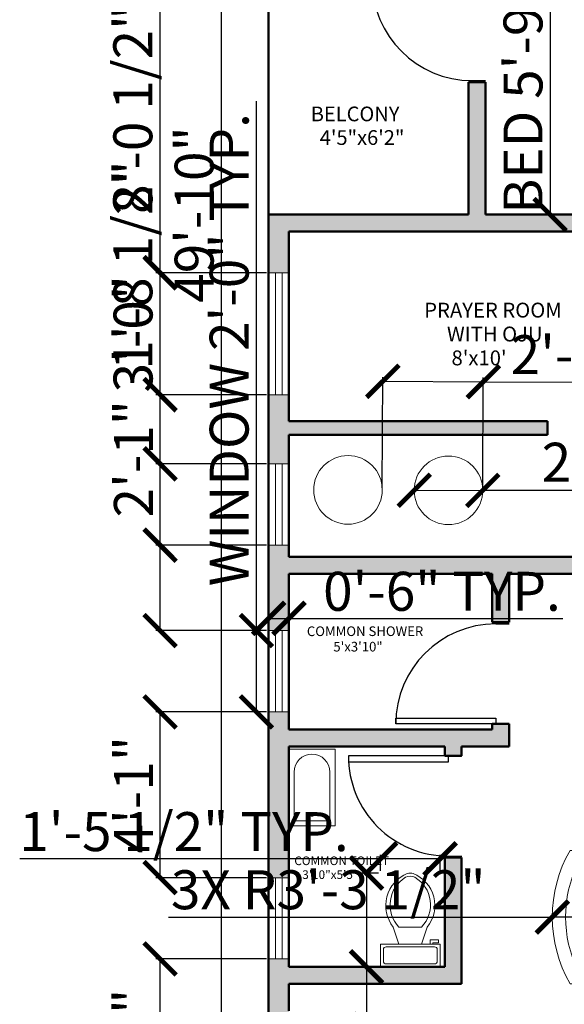
# Model space of a CAD drawing. Units: inches. Extents: x 3147 to 3847, y 1414 to 2207.
# Tile 2 of 7: x 3276 to 3437, y 1561 to 1852. Entities that reach past the tile are written whole.
import ezdxf

# ---------------------------------------------------------------- set-up
doc = ezdxf.new("R2010")
doc.units = ezdxf.units.IN
for name, color, linetype, lineweight in [('A-ANNO-DIMS', 2, 'Continuous', 18), ('A-AREA-IDEN', 7, 'Continuous', 18), ('A-DOOR', 3, 'Continuous', 25), ('A-FLOR-FIXT', 9, 'Continuous', 18), ('A-FURN', 8, 'Continuous', 18), ('A-GLAZ', 4, 'Continuous', 18), ('A-WALL', 7, 'Continuous', 50)]:
    doc.layers.add(name, color=color, linetype=linetype, lineweight=lineweight)
doc.layers.add('A-WALL-PATT', color=18, linetype='Continuous', lineweight=13, true_color=0x000000)
doc.styles.get("Standard").update_dxf_attribs({"font": 'arial.ttf'})
doc.dimstyles.new('ISO-25', dxfattribs={"dimtxt": 11.5, "dimasz": 9.5, "dimexe": 1.25, "dimexo": 0.625, "dimtad": 1, "dimdec": 0, "dimlunit": 3, "dimtxsty": 'Standard', "dimblk": 'ARCHTICK', "dimcen": 2.5, "dimadec": 0, "dimazin": 0, "dimtfac": 1, "dimtdec": 0, "dimtmove": 0, "dimatfit": 3, "dimfxl": 1, "dimarcsym": 0})

# ---------------------------------------------------------------- blocks, each defined once
blk = doc.blocks.new('*U3')
for p, q in [((0, 0), (0, -100)), ((750, 0), (750, -100))]:
    blk.add_line(p, q)
blk.add_lwpolyline([(0, 0), (0, 750), (43.75, 750), (43.75, 0)], close=True)
blk.add_arc((0, 0), 750, 0, 90)
blk = doc.blocks.new('*U4')
for p, q in [((-750, 0), (-750, -100)), ((0, 0), (0, -100))]:
    blk.add_line(p, q)
blk.add_lwpolyline([(0, 0), (0, 750), (-43.75, 750), (-43.75, 0)], close=True)
blk.add_arc((0, 0), 750, 90, 180)
blk = doc.blocks.new('Bath Tub - 26 x 60 in.')
for p, q in [((8, -18), (10, -18)), ((9, -17), (9, -19))]:
    blk.add_line(p, q)
blk.add_lwpolyline([(0, -36), (0, 0), (60, 0), (60, -36)], close=True)
for points in [[(4, -30), (4, -6)], [(6, -4), (42, -4)], [(42, -32), (6, -32)]]:
    blk.add_lwpolyline(points)
for radius in [1.5, 1]:
    blk.add_circle((9, -18), radius)
for centre, radius, start, end in [((5.75, -5.75), 1.77, 81.8699, 188.1301), ((42, -18), 14, 270, 90), ((5.75, -30.25), 1.77, 171.8699, 278.1301)]:
    blk.add_arc(centre, radius, start, end)
blk = doc.blocks.new('Toilet - top')
for p, q in [((9.5, -6), (9.5, -2)), ((-10, -8.5), (-8, -8.5)), ((-10, -9.5), (-10, -8.5)), ((-7, -9.5), (-10, -9.5)), ((-8, -8.5), (-8, -8)), ((-7, -8), (-7, -9.5)), ((-4, -8), (-6, -14)), ((4, -8), (6, -14)), ((4, -14), (-4, -14))]:
    blk.add_line(p, q)
blk.add_lwpolyline([(10.5, -8), (10.5, 0), (-10.5, 0), (-10.5, -8)], close=True)
for points in [[(-9.5, -2), (-9.5, -6)], [(8.5, -1), (-8.5, -1)], [(-8.5, -7), (8.5, -7)]]:
    blk.add_lwpolyline(points)
for centre, radius, start, end in [((-8.62, -1.88), 0.884, 81.8699, 188.1301), ((8.62, -1.88), 0.884, 351.8699, 98.1301), ((-8.62, -6.12), 0.884, 171.8699, 278.1301), ((8.62, -6.12), 0.884, 261.8699, 8.1301), ((3.52, -21.58), 12.17, 141.4691, 247.9714), ((4.2, -21.82), 11.33, 136.3677, 238.9468), ((-3.52, -21.58), 12.17, 292.0284, 38.5307), ((-4.2, -21.82), 11.33, 301.053, 43.6321), ((0, -27.88), 4, 245.7318, 294.2682), ((0, -29), 4, 254.8605, 285.1395)]:
    blk.add_arc(centre, radius, start, end)
blk = doc.blocks.new('Sofa - Roundback Loveseat 5 ft.')
for p, q in [((0, -32.44198), (0, -5.99998)), ((-24, -33.99998), (-24, -11.46958)), ((24.00004, -33.99998), (24.00004, -11.46958)), ((-23.9998, -13.38178), (23.99986, -13.38178)), ((-24, -32.44198), (24.00004, -32.44198))]:
    blk.add_line(p, q)
for points in [[(-24, -33.99998), (-30, -33.99998), (-30, -7.99998)], [(30.00004, -7.99998), (30.00004, -33.99998), (24.00004, -33.99998)]]:
    blk.add_lwpolyline(points)
for centre, radius, start, end in [((0, -60.24998), 60.24998, 60.13715, 119.8628), ((0, -61.38438), 55.38444, 64.32083, 115.6792)]:
    blk.add_arc(centre, radius, start, end)
blk = doc.blocks.new('_ArchTick')
at = {"color": 0, "linetype": 'ByBlock', "const_width": 0.15}
blk.add_lwpolyline([(-0.5, -0.5), (0.5, 0.5)], dxfattribs=at)
blk = doc.blocks.new('*D22')
at = {"layer": 'A-ANNO-DIMS', "color": 0, "lineweight": -2, "transparency": 16777216}
for p, q in [((3349.14, 2093.05), (3334.5, 2093.05)), ((3335.75, 2093.05), (3335.75, 1495.05)), ((3349.14, 1495.05), (3334.5, 1495.05))]:
    blk.add_line(p, q, dxfattribs=at)
at = {"layer": 'Defpoints', "color": 0, "transparency": 16777216}
for p in [(3349.76, 2093.05), (3335.75, 1495.05), (3349.76, 1495.05)]:
    blk.add_point(p, dxfattribs=at)
at = {"layer": 'A-ANNO-DIMS', "color": 0, "lineweight": -2, "transparency": 16777216, "xscale": 9.5, "yscale": 9.5, "zscale": 9.5}
for p, rotation in [((3335.75, 2093.05), 90), ((3335.75, 1495.05), 270)]:
    blk.add_blockref('_ArchTick', p, dxfattribs=dict(at, rotation=rotation))
at = {"layer": 'A-ANNO-DIMS', "color": 0, "transparency": 16777216, "insert": (3329.25, 1794.05), "char_height": 11.5, "attachment_point": 5, "rotation": 90}
blk.add_mtext('49\'-10"', dxfattribs=at)
blk = doc.blocks.new('WIN-24IN')
for p, q in [((6, 24), (0, 24)), ((2, 0), (2, 24)), ((4, 0), (4, 24)), ((6, 0), (0, 0))]:
    blk.add_line(p, q)
blk = doc.blocks.new('OJU-ROUND-FIXTURE')
blk.add_circle((10.13, 10.13), 10.13)
blk = doc.blocks.new('*D27')
at = {"layer": 'A-ANNO-DIMS', "color": 0, "lineweight": -2, "transparency": 16777216}
for p, q in [((3346.16, 1671.27), (3346.16, 1827.54)), ((3349.14, 1671.27), (3344.91, 1671.27)), ((3346.16, 1647.27), (3346.16, 1671.27)), ((3349.14, 1647.27), (3344.91, 1647.27))]:
    blk.add_line(p, q, dxfattribs=at)
at = {"layer": 'Defpoints', "color": 0, "transparency": 16777216}
for p in [(3346.16, 1671.27), (3349.76, 1671.27), (3349.76, 1647.27)]:
    blk.add_point(p, dxfattribs=at)
at = {"layer": 'A-ANNO-DIMS', "color": 0, "lineweight": -2, "transparency": 16777216, "xscale": 9.5, "yscale": 9.5, "zscale": 9.5}
for p, rotation in [((3346.16, 1671.27), 90), ((3346.16, 1647.27), 270)]:
    blk.add_blockref('_ArchTick', p, dxfattribs=dict(at, rotation=rotation))
at = {"layer": 'A-ANNO-DIMS', "color": 0, "transparency": 16777216, "insert": (3339.59, 1754.16), "char_height": 11.5, "attachment_point": 5, "rotation": 90}
blk.add_mtext('WINDOW 2\'-0" TYP.', dxfattribs=at)
blk = doc.blocks.new('*D28')
at = {"layer": 'A-ANNO-DIMS', "color": 0, "lineweight": -2, "transparency": 16777216}
for p, q in [((3349.76, 1671.9), (3349.76, 1676.12)), ((3349.76, 1674.87), (3355.76, 1674.87)), ((3355.76, 1671.9), (3355.76, 1676.12)), ((3355.76, 1674.87), (3436.61, 1674.87))]:
    blk.add_line(p, q, dxfattribs=at)
at = {"layer": 'Defpoints', "color": 0, "transparency": 16777216}
for p in [(3355.76, 1674.87), (3349.76, 1671.27), (3355.76, 1671.27)]:
    blk.add_point(p, dxfattribs=at)
at = {"layer": 'A-ANNO-DIMS', "color": 0, "lineweight": -2, "transparency": 16777216, "xscale": 9.5, "yscale": 9.5, "zscale": 9.5, "rotation": 180}
blk.add_blockref('_ArchTick', (3349.76, 1674.87), dxfattribs=at)
at = {"layer": 'A-ANNO-DIMS', "color": 0, "lineweight": -2, "transparency": 16777216, "xscale": 9.5, "yscale": 9.5, "zscale": 9.5}
blk.add_blockref('_ArchTick', (3355.76, 1674.87), dxfattribs=at)
at = {"layer": 'A-ANNO-DIMS', "color": 0, "transparency": 16777216, "insert": (3400.94, 1681.37), "char_height": 11.5, "attachment_point": 5}
blk.add_mtext('0\'-6" TYP.', dxfattribs=at)
blk = doc.blocks.new('*D31')
at = {"layer": 'A-ANNO-DIMS', "color": 0, "lineweight": -2, "transparency": 16777216}
for p, q in [((3382.17, 1599.72), (3377.4, 1599.72)), ((3378.65, 1599.72), (3378.65, 1572.05)), ((3382.17, 1572.05), (3377.4, 1572.05)), ((3378.65, 1572.05), (3378.65, 1432.7))]:
    blk.add_line(p, q, dxfattribs=at)
at = {"layer": 'Defpoints', "color": 0, "transparency": 16777216}
for p in [(3382.8, 1599.72), (3378.65, 1572.05), (3382.8, 1572.05)]:
    blk.add_point(p, dxfattribs=at)
at = {"layer": 'A-ANNO-DIMS', "color": 0, "lineweight": -2, "transparency": 16777216, "xscale": 9.5, "yscale": 9.5, "zscale": 9.5}
for p, rotation in [((3378.65, 1599.72), 90), ((3378.65, 1572.05), 270)]:
    blk.add_blockref('_ArchTick', p, dxfattribs=dict(at, rotation=rotation))
at = {"layer": 'A-ANNO-DIMS', "color": 0, "transparency": 16777216, "insert": (3372.07, 1497.63), "char_height": 11.5, "attachment_point": 5, "rotation": 90}
blk.add_mtext('WC 2\'-3 1/2" TYP.', dxfattribs=at)
blk = doc.blocks.new('*D32')
at = {"layer": 'A-ANNO-DIMS', "color": 0, "lineweight": -2, "transparency": 16777216}
for p, q in [((3382.8, 1600.35), (3382.8, 1605.13)), ((3400.39, 1600.35), (3400.39, 1605.13)), ((3382.8, 1603.88), (3276.24, 1603.88)), ((3400.39, 1603.88), (3382.8, 1603.88))]:
    blk.add_line(p, q, dxfattribs=at)
at = {"layer": 'Defpoints', "color": 0, "transparency": 16777216}
for p in [(3382.8, 1603.88), (3382.8, 1599.72), (3400.39, 1599.72)]:
    blk.add_point(p, dxfattribs=at)
at = {"layer": 'A-ANNO-DIMS', "color": 0, "lineweight": -2, "transparency": 16777216, "xscale": 9.5, "yscale": 9.5, "zscale": 9.5, "rotation": 180}
blk.add_blockref('_ArchTick', (3382.8, 1603.88), dxfattribs=at)
at = {"layer": 'A-ANNO-DIMS', "color": 0, "lineweight": -2, "transparency": 16777216, "xscale": 9.5, "yscale": 9.5, "zscale": 9.5}
blk.add_blockref('_ArchTick', (3400.39, 1603.88), dxfattribs=at)
at = {"layer": 'A-ANNO-DIMS', "color": 0, "transparency": 16777216, "insert": (3324.77, 1610.45), "char_height": 11.5, "attachment_point": 5}
blk.add_mtext('1\'-5 1/2" TYP.', dxfattribs=at)
blk = doc.blocks.new('*D35')
at = {"layer": 'A-ANNO-DIMS', "color": 0, "lineweight": -2, "transparency": 16777216}
for p, q in [((3442.6, 1863.12), (3431.61, 1863.12)), ((3432.86, 1863.12), (3432.86, 1794.05)), ((3442.6, 1794.05), (3431.61, 1794.05))]:
    blk.add_line(p, q, dxfattribs=at)
at = {"layer": 'Defpoints', "color": 0, "transparency": 16777216}
for p in [(3443.22, 1863.12), (3432.86, 1794.05), (3443.22, 1794.05)]:
    blk.add_point(p, dxfattribs=at)
at = {"layer": 'A-ANNO-DIMS', "color": 0, "lineweight": -2, "transparency": 16777216, "xscale": 9.5, "yscale": 9.5, "zscale": 9.5}
for p, rotation in [((3432.86, 1863.12), 90), ((3432.86, 1794.05), 270)]:
    blk.add_blockref('_ArchTick', p, dxfattribs=dict(at, rotation=rotation))
at = {"layer": 'A-ANNO-DIMS', "color": 0, "transparency": 16777216, "insert": (3426.36, 1828.59), "char_height": 11.5, "attachment_point": 5, "rotation": 90}
blk.add_mtext('BED 5\'-9"', dxfattribs=at)
blk = doc.blocks.new('*D51')
at = {"layer": 'A-ANNO-DIMS', "color": 0, "lineweight": -2, "transparency": 16777216}
for p, q in [((3383.32, 1713.42), (3383.48, 1746.09)), ((3383.47, 1744.84), (3413.15, 1744.7)), ((3413, 1713.28), (3413.15, 1745.95)), ((3413.15, 1744.7), (3481.46, 1744.38))]:
    blk.add_line(p, q, dxfattribs=at)
at = {"layer": 'Defpoints', "color": 0, "transparency": 16777216}
for p in [(3413.15, 1744.7), (3383.32, 1712.8), (3412.99, 1712.65)]:
    blk.add_point(p, dxfattribs=at)
at = {"layer": 'A-ANNO-DIMS', "color": 0, "lineweight": -2, "transparency": 16777216, "xscale": 9.5, "yscale": 9.5, "zscale": 9.5}
for p, rotation in [((3383.47, 1744.84), 179.7281677872788), ((3413.15, 1744.7), 359.7281677872788)]:
    blk.add_blockref('_ArchTick', p, dxfattribs=dict(at, rotation=rotation))
at = {"layer": 'A-ANNO-DIMS', "color": 0, "transparency": 16777216, "insert": (3452.08, 1751.09), "char_height": 11.5, "attachment_point": 5, "rotation": 359.7282}
blk.add_mtext('2\'-5 1/2"', dxfattribs=at)
blk = doc.blocks.new('*D75')
at = {"layer": 'A-ANNO-DIMS', "color": 0, "lineweight": -2, "transparency": 16777216}
for p, q in [((3349.14, 1574.35), (3316.46, 1574.35)), ((3317.71, 1495.05), (3317.71, 1574.35)), ((3349.14, 1495.05), (3316.46, 1495.05))]:
    blk.add_line(p, q, dxfattribs=at)
at = {"layer": 'Defpoints', "color": 0, "transparency": 16777216}
for p in [(3317.71, 1574.35), (3349.76, 1574.35), (3349.76, 1495.05)]:
    blk.add_point(p, dxfattribs=at)
at = {"layer": 'A-ANNO-DIMS', "color": 0, "lineweight": -2, "transparency": 16777216, "xscale": 9.5, "yscale": 9.5, "zscale": 9.5}
for p, rotation in [((3317.71, 1574.35), 90), ((3317.71, 1495.05), 270)]:
    blk.add_blockref('_ArchTick', p, dxfattribs=dict(at, rotation=rotation))
at = {"layer": 'A-ANNO-DIMS', "color": 0, "transparency": 16777216, "insert": (3311.14, 1534.7), "char_height": 11.5, "attachment_point": 5, "rotation": 90}
blk.add_mtext('6\'-7 1/2"', dxfattribs=at)
blk = doc.blocks.new('*D76')
at = {"layer": 'A-ANNO-DIMS', "color": 0, "lineweight": -2, "transparency": 16777216}
for p, q in [((3349.14, 1647.27), (3316.46, 1647.27)), ((3317.71, 1598.35), (3317.71, 1647.27)), ((3349.14, 1598.35), (3316.46, 1598.35))]:
    blk.add_line(p, q, dxfattribs=at)
at = {"layer": 'Defpoints', "color": 0, "transparency": 16777216}
for p in [(3317.71, 1647.27), (3349.76, 1647.27), (3349.76, 1598.35)]:
    blk.add_point(p, dxfattribs=at)
at = {"layer": 'A-ANNO-DIMS', "color": 0, "lineweight": -2, "transparency": 16777216, "xscale": 9.5, "yscale": 9.5, "zscale": 9.5}
for p, rotation in [((3317.71, 1647.27), 90), ((3317.71, 1598.35), 270)]:
    blk.add_blockref('_ArchTick', p, dxfattribs=dict(at, rotation=rotation))
at = {"layer": 'A-ANNO-DIMS', "color": 0, "transparency": 16777216, "insert": (3311.32, 1622.81), "char_height": 11.5, "attachment_point": 5, "rotation": 90}
blk.add_mtext('4\'-1"', dxfattribs=at)
blk = doc.blocks.new('*D77')
at = {"layer": 'A-ANNO-DIMS', "color": 0, "lineweight": -2, "transparency": 16777216}
for p, q in [((3317.71, 1696.47), (3317.71, 1737.98)), ((3349.14, 1696.47), (3316.46, 1696.47)), ((3317.71, 1671.27), (3317.71, 1696.47)), ((3349.14, 1671.27), (3316.46, 1671.27))]:
    blk.add_line(p, q, dxfattribs=at)
at = {"layer": 'Defpoints', "color": 0, "transparency": 16777216}
for p in [(3317.71, 1696.47), (3349.76, 1696.47), (3349.76, 1671.27)]:
    blk.add_point(p, dxfattribs=at)
at = {"layer": 'A-ANNO-DIMS', "color": 0, "lineweight": -2, "transparency": 16777216, "xscale": 9.5, "yscale": 9.5, "zscale": 9.5}
for p, rotation in [((3317.71, 1696.47), 90), ((3317.71, 1671.27), 270)]:
    blk.add_blockref('_ArchTick', p, dxfattribs=dict(at, rotation=rotation))
at = {"layer": 'A-ANNO-DIMS', "color": 0, "transparency": 16777216, "insert": (3311.32, 1721.98), "char_height": 11.5, "attachment_point": 5, "rotation": 90}
blk.add_mtext('2\'-1"', dxfattribs=at)
blk = doc.blocks.new('*D78')
at = {"layer": 'A-ANNO-DIMS', "color": 0, "lineweight": -2, "transparency": 16777216}
for p, q in [((3317.71, 1740.88), (3317.71, 1807.92)), ((3349.14, 1740.88), (3316.46, 1740.88)), ((3317.71, 1720.47), (3317.71, 1740.88)), ((3349.14, 1720.47), (3316.46, 1720.47))]:
    blk.add_line(p, q, dxfattribs=at)
at = {"layer": 'Defpoints', "color": 0, "transparency": 16777216}
for p in [(3317.71, 1740.88), (3349.76, 1740.88), (3349.76, 1720.47)]:
    blk.add_point(p, dxfattribs=at)
at = {"layer": 'A-ANNO-DIMS', "color": 0, "lineweight": -2, "transparency": 16777216, "xscale": 9.5, "yscale": 9.5, "zscale": 9.5}
for p, rotation in [((3317.71, 1740.88), 90), ((3317.71, 1720.47), 270)]:
    blk.add_blockref('_ArchTick', p, dxfattribs=dict(at, rotation=rotation))
at = {"layer": 'A-ANNO-DIMS', "color": 0, "transparency": 16777216, "insert": (3311.14, 1779.15), "char_height": 11.5, "attachment_point": 5, "rotation": 90}
blk.add_mtext('1\'-8 1/2"', dxfattribs=at)
blk = doc.blocks.new('*D79')
at = {"layer": 'A-ANNO-DIMS', "color": 0, "lineweight": -2, "transparency": 16777216}
for p, q in [((3349.14, 1776.88), (3316.46, 1776.88)), ((3317.71, 1740.88), (3317.71, 1776.88)), ((3349.14, 1740.88), (3316.46, 1740.88))]:
    blk.add_line(p, q, dxfattribs=at)
at = {"layer": 'Defpoints', "color": 0, "transparency": 16777216}
for p in [(3317.71, 1776.88), (3349.76, 1776.88), (3349.76, 1740.88)]:
    blk.add_point(p, dxfattribs=at)
at = {"layer": 'A-ANNO-DIMS', "color": 0, "lineweight": -2, "transparency": 16777216, "xscale": 9.5, "yscale": 9.5, "zscale": 9.5}
for p, rotation in [((3317.71, 1776.88), 90), ((3317.71, 1740.88), 270)]:
    blk.add_blockref('_ArchTick', p, dxfattribs=dict(at, rotation=rotation))
at = {"layer": 'A-ANNO-DIMS', "color": 0, "transparency": 16777216, "insert": (3311.21, 1758.88), "char_height": 11.5, "attachment_point": 5, "rotation": 90}
blk.add_mtext('3\'-0"', dxfattribs=at)
blk = doc.blocks.new('*D80')
at = {"layer": 'A-ANNO-DIMS', "color": 0, "lineweight": -2, "transparency": 16777216}
for p, q in [((3349.14, 1873.34), (3316.46, 1873.34)), ((3317.71, 1776.88), (3317.71, 1873.34)), ((3349.14, 1776.88), (3316.46, 1776.88))]:
    blk.add_line(p, q, dxfattribs=at)
at = {"layer": 'Defpoints', "color": 0, "transparency": 16777216}
for p in [(3317.71, 1873.34), (3349.76, 1873.34), (3349.76, 1776.88)]:
    blk.add_point(p, dxfattribs=at)
at = {"layer": 'A-ANNO-DIMS', "color": 0, "lineweight": -2, "transparency": 16777216, "xscale": 9.5, "yscale": 9.5, "zscale": 9.5}
for p, rotation in [((3317.71, 1873.34), 90), ((3317.71, 1776.88), 270)]:
    blk.add_blockref('_ArchTick', p, dxfattribs=dict(at, rotation=rotation))
at = {"layer": 'A-ANNO-DIMS', "color": 0, "transparency": 16777216, "insert": (3311.14, 1825.11), "char_height": 11.5, "attachment_point": 5, "rotation": 90}
blk.add_mtext('8\'-0 1/2"', dxfattribs=at)
blk = doc.blocks.new('*D94')
at = {"layer": 'A-ANNO-DIMS', "color": 0, "lineweight": -2, "transparency": 16777216}
for p in [(3392.74, 1712.66), (3527.42, 1712.6)]:
    blk.add_line(p, (3412.99, 1712.65), dxfattribs=at)
at = {"layer": 'Defpoints', "color": 0, "transparency": 16777216}
for p in [(3392.74, 1712.66), (3412.99, 1712.65)]:
    blk.add_point(p, dxfattribs=at)
at = {"layer": 'A-ANNO-DIMS', "color": 0, "lineweight": -2, "transparency": 16777216, "xscale": 9.5, "yscale": 9.5, "zscale": 9.5}
for p, rotation in [((3392.74, 1712.66), 359.9757507078119), ((3412.99, 1712.65), 179.9757507078119)]:
    blk.add_blockref('_ArchTick', p, dxfattribs=dict(at, rotation=rotation))
at = {"layer": 'A-ANNO-DIMS', "color": 0, "transparency": 16777216, "insert": (3479.71, 1719.44), "char_height": 11.5, "attachment_point": 5, "rotation": 359.9758}
blk.add_mtext('2X ∅1\'-8 1/2"', dxfattribs=at)
blk = doc.blocks.new('*D97')
at = {"layer": 'A-ANNO-DIMS', "color": 0, "lineweight": -2, "transparency": 16777216}
for p in [(3320.2, 1586.73), (3473.05, 1586.73)]:
    blk.add_line(p, (3433.52, 1586.73), dxfattribs=at)
at = {"layer": 'Defpoints', "color": 0, "transparency": 16777216}
for p in [(3433.52, 1586.73), (3473.05, 1586.73)]:
    blk.add_point(p, dxfattribs=at)
at = {"layer": 'A-ANNO-DIMS', "color": 0, "lineweight": -2, "transparency": 16777216, "xscale": 9.5, "yscale": 9.5, "zscale": 9.5, "rotation": 359.9999231677337}
blk.add_blockref('_ArchTick', (3433.52, 1586.73), dxfattribs=at)
at = {"layer": 'A-ANNO-DIMS', "color": 0, "transparency": 16777216, "insert": (3367.36, 1593.3), "char_height": 11.5, "attachment_point": 5, "rotation": 359.9999}
blk.add_mtext('3X R3\'-3 1/2"', dxfattribs=at)

msp = doc.modelspace()

# ---------------------------------------------------------------- hatches: boundary and pattern name
at = {"layer": 'A-WALL-PATT'}
h = msp.add_hatch(color=256, dxfattribs=at)
h.dxf.hatch_style = 1
h.paths.add_polyline_path([(3616.76, 2093.05), (3594.02, 2093.05), (3594.02, 2087.05), (3611.76, 2087.05), (3611.76, 1993.05), (3616.76, 1993.05), (3628.76, 1993.05), (3628.76, 1996.99), (3628.76, 1998.05), (3616.76, 1998.05), (3616.76, 2087.05)])
h.paths.add_polyline_path([(3576.44, 2093.05), (3527.03, 2093.05), (3527.03, 2087.05), (3546.76, 2087.05), (3546.76, 1962.05), (3551.76, 1962.05), (3590.76, 1962.05), (3590.76, 1921.05), (3585.76, 1921.05), (3585.76, 1916.05), (3590.76, 1916.05), (3590.76, 1895.05), (3595.76, 1895.05), (3595.76, 1962.05), (3611.76, 1962.05), (3616.76, 1962.05), (3616.76, 1969.05), (3611.76, 1969.05), (3611.76, 1967.05), (3551.76, 1967.05), (3551.76, 2087.05), (3576.44, 2087.05)])
h.paths.add_polyline_path([(3455.03, 2093.05), (3408.76, 2093.05), (3408.76, 2087.05), (3408.76, 2046.06), (3413.76, 2046.06), (3413.76, 2087.05), (3455.03, 2087.05)])
h.paths.add_polyline_path([(3355.76, 2008.05), (3408.76, 2008.05), (3408.76, 2004.83), (3413.76, 2004.83), (3413.76, 2008.05), (3413.76, 2013.05), (3413.76, 2016.06), (3408.76, 2016.06), (3408.76, 2013.05), (3355.76, 2013.05), (3349.76, 2013.05), (3349.76, 1973.71), (3355.76, 1973.71)])
h.paths.add_polyline_path([(3413.76, 1974.83), (3408.76, 1974.83), (3408.76, 1943.05), (3355.76, 1943.05), (3355.76, 1949.71), (3349.76, 1949.71), (3349.76, 1897.34), (3355.76, 1897.34), (3355.76, 1938.05), (3408.76, 1938.05), (3408.76, 1934.63), (3413.76, 1934.63), (3413.76, 1938.05), (3505.76, 1938.05), (3505.76, 1916.05), (3533.76, 1916.05), (3533.76, 1904.63), (3533.76, 1831.83), (3538.76, 1831.83), (3538.76, 1904.63), (3538.76, 1916.05), (3546.76, 1916.05), (3549.76, 1916.05), (3549.76, 1921.05), (3546.76, 1921.05), (3510.76, 1921.05), (3510.76, 1938.05), (3510.76, 1943.05), (3413.76, 1943.05)])
h.paths.add_polyline_path([(3413.76, 1904.63), (3408.76, 1904.63), (3408.76, 1870.05), (3355.76, 1870.05), (3355.76, 1873.34), (3349.76, 1873.34), (3349.76, 1865.05), (3355.76, 1865.05), (3408.76, 1865.05), (3408.76, 1863.11), (3409.83, 1863.11), (3413.76, 1863.11)], flags=17)
h.paths.add_polyline_path([(3538.76, 1795.83), (3533.76, 1795.83), (3533.76, 1794.05), (3413.76, 1794.05), (3413.76, 1833.11), (3408.76, 1833.11), (3408.76, 1794.05), (3355.76, 1794.05), (3349.76, 1794.05), (3349.76, 1776.88), (3355.76, 1776.88), (3355.76, 1789.05), (3413.76, 1789.05), (3475.76, 1789.05), (3475.76, 1731.91), (3480.76, 1731.91), (3480.76, 1789.05), (3538.76, 1789.05)])
h.paths.add_polyline_path([(3432.14, 1733.05), (3413.76, 1733.05), (3355.76, 1733.05), (3355.76, 1740.88), (3349.76, 1740.88), (3349.76, 1720.47), (3355.76, 1720.47), (3355.76, 1729.05), (3413.76, 1729.05), (3432.14, 1729.05)])
h.paths.add_polyline_path([(3480.76, 1695.91), (3476.83, 1695.91), (3475.76, 1695.91), (3475.76, 1693.05), (3413.76, 1693.05), (3355.76, 1693.05), (3355.76, 1696.47), (3349.76, 1696.47), (3349.76, 1671.27), (3355.76, 1671.27), (3355.76, 1688.05), (3413.76, 1688.05), (3415.76, 1688.05), (3415.76, 1673.71), (3420.76, 1673.71), (3420.76, 1688.05), (3480.76, 1688.05)])
h.paths.add_polyline_path([(3420.76, 1643.71), (3415.76, 1643.71), (3415.76, 1642.05), (3413.76, 1642.05), (3355.76, 1642.05), (3355.76, 1647.27), (3349.76, 1647.27), (3349.76, 1598.35), (3355.76, 1598.35), (3355.76, 1637.05), (3401.76, 1637.05), (3401.76, 1634.26), (3406.76, 1634.26), (3406.76, 1637.05), (3413.76, 1637.05), (3420.76, 1637.05)])
h.paths.add_polyline_path([(3406.76, 1604.26), (3401.76, 1604.26), (3401.76, 1572.05), (3355.76, 1572.05), (3355.76, 1574.35), (3349.76, 1574.35), (3349.76, 1553.05), (3349.76, 1495.05), (3371.89, 1495.05), (3371.89, 1501.05), (3355.76, 1501.05), (3355.76, 1559.05), (3355.76, 1567.05), (3406.76, 1567.05), (3406.76, 1572.05)])
h.paths.add_polyline_path([(3534.41, 1501.05), (3419.89, 1501.05), (3419.89, 1495.05), (3534.41, 1495.05)])
h.paths.add_polyline_path([(3769.76, 1509.48), (3763.76, 1509.48), (3763.76, 1501.05), (3600.76, 1501.05), (3600.76, 1548.51), (3595.76, 1548.51), (3595.76, 1501.05), (3582.41, 1501.05), (3582.41, 1495.05), (3769.76, 1495.05)])
h.paths.add_polyline_path([(3769.76, 1645.82), (3763.76, 1645.82), (3763.76, 1593.05), (3664.76, 1593.05), (3619.76, 1593.05), (3619.76, 1674.05), (3614.76, 1674.05), (3614.76, 1593.05), (3595.76, 1593.05), (3595.76, 1584.51), (3600.76, 1584.51), (3600.76, 1588.05), (3619.76, 1588.05), (3664.76, 1588.05), (3763.76, 1588.05), (3763.76, 1569.48), (3769.76, 1569.48)])
h.paths.add_polyline_path([(3769.76, 1731.24), (3763.76, 1731.24), (3763.76, 1718.05), (3664.76, 1718.05), (3595.76, 1718.05), (3595.76, 1723.05), (3590.76, 1723.05), (3590.76, 1713.05), (3595.76, 1713.05), (3614.76, 1713.05), (3614.76, 1710.05), (3619.76, 1710.05), (3619.76, 1713.05), (3664.76, 1713.05), (3763.76, 1713.05), (3763.76, 1693.82), (3769.76, 1693.82)])
h.paths.add_polyline_path([(3769.76, 1872.64), (3763.76, 1872.64), (3763.76, 1854.05), (3664.76, 1854.05), (3595.76, 1854.05), (3595.76, 1859.05), (3590.76, 1859.05), (3590.76, 1759.05), (3595.76, 1759.05), (3595.76, 1849.05), (3664.76, 1849.05), (3763.76, 1849.05), (3763.76, 1815.24), (3769.76, 1815.24)])
h.paths.add_polyline_path([(3769.76, 1998.05), (3763.76, 1998.05), (3763.76, 1968.64), (3769.76, 1968.64)])
h.paths.add_polyline_path([(3763.76, 1998.05), (3664.76, 1998.05), (3664.76, 1993.05), (3763.76, 1993.05)])

# ---------------------------------------------------------------- linework, layer by layer
at = {"layer": 'A-GLAZ'}
for p, q in [((3355.76, 1776.88), (3349.76, 1776.88)), ((3351.76, 1740.88), (3351.76, 1776.88)), ((3353.76, 1740.88), (3353.76, 1776.88)), ((3355.76, 1740.88), (3349.76, 1740.88))]:
    msp.add_line(p, q, dxfattribs=at)
at = {"layer": 'A-WALL'}
for p, q in [((3349.76, 1553.05), (3349.76, 2093.05)), ((3408.76, 1794.05), (3408.76, 1833.11)), ((3408.76, 1833.11), (3413.76, 1833.11)), ((3413.76, 1794.05), (3413.76, 1833.11)), ((3355.76, 1794.05), (3349.76, 1794.05)), ((3355.76, 1733.05), (3355.76, 1789.05)), ((3432.14, 1729.05), (3432.14, 1733.05)), ((3355.76, 1693.05), (3355.76, 1729.05)), ((3355.76, 1642.05), (3355.76, 1688.05)), ((3415.76, 1673.71), (3415.76, 1688.05)), ((3420.76, 1673.71), (3420.76, 1688.05)), ((3415.76, 1673.71), (3420.76, 1673.71)), ((3415.76, 1642.05), (3415.76, 1643.71)), ((3415.76, 1643.71), (3420.76, 1643.71)), ((3420.76, 1637.05), (3420.76, 1643.71)), ((3355.76, 1572.05), (3355.76, 1637.05)), ((3401.76, 1634.26), (3401.76, 1637.05)), ((3406.76, 1634.26), (3406.76, 1637.05)), ((3406.76, 1634.26), (3401.76, 1634.26)), ((3401.76, 1572.05), (3401.76, 1604.26)), ((3406.76, 1604.26), (3401.76, 1604.26)), ((3406.76, 1572.05), (3406.76, 1604.26)), ((3406.76, 1572.05), (3406.76, 1567.05)), ((3355.76, 1559.05), (3355.76, 1567.05))]:
    msp.add_line(p, q, dxfattribs=at)
for points in [[(3408.76, 1794.05), (3355.76, 1794.05)], [(3533.76, 1794.05), (3413.76, 1794.05)], [(3475.76, 1789.05), (3413.76, 1789.05), (3355.76, 1789.05)], [(3432.14, 1733.05), (3413.76, 1733.05), (3355.76, 1733.05)], [(3432.14, 1729.05), (3413.76, 1729.05), (3355.76, 1729.05)], [(3475.76, 1695.91), (3475.76, 1693.05), (3413.76, 1693.05), (3355.76, 1693.05)], [(3480.76, 1695.91), (3480.76, 1688.05), (3420.76, 1688.05)], [(3415.76, 1688.05), (3413.76, 1688.05), (3355.76, 1688.05)], [(3415.76, 1642.05), (3413.76, 1642.05), (3355.76, 1642.05)], [(3401.76, 1637.05), (3355.76, 1637.05)], [(3420.76, 1637.05), (3413.76, 1637.05), (3406.76, 1637.05)], [(3401.76, 1572.05), (3355.76, 1572.05)], [(3406.76, 1567.05), (3355.76, 1567.05)]]:
    msp.add_lwpolyline(points, dxfattribs=at)

# ---------------------------------------------------------------- block references
at = {"layer": 'A-DOOR', "xscale": 0.0393700787401575, "yscale": 0.0393700787401575, "zscale": 0.0393700787401575}
for name, p, rotation in [('*U4', (3409.83, 1863.11), 90), ('*U3', (3416.83, 1643.71), 89.99999999999999), ('*U4', (3402.83, 1634.26), 89.99999999999999)]:
    msp.add_blockref(name, p, dxfattribs=dict(at, rotation=rotation))
at = {"layer": 'A-FLOR-FIXT'}
for p in [(3363.07, 1702.67), (3392.74, 1702.53)]:
    msp.add_blockref('OJU-ROUND-FIXTURE', p, dxfattribs=at)
for name, p, xscale, yscale, zscale, rotation in [('Bath Tub - 26 x 60 in.', (3355.76, 1613.62), 0.3777777777777778, 0.3777777777777778, 0.3777777777777778, 90), ('Toilet - top', (3391.59, 1572.05), 0.8374824719350153, 0.8374824719350153, 0.8374824719350153, 180)]:
    msp.add_blockref(name, p, dxfattribs=dict(at, xscale=xscale, yscale=yscale, zscale=zscale, rotation=rotation))
at = {"layer": 'A-FURN', "xscale": 0.6559911100175418, "yscale": 0.6559911100175418, "zscale": 0.6559911100175418, "rotation": 90}
msp.add_blockref('Sofa - Roundback Loveseat 5 ft.', (3433.52, 1586.73), dxfattribs=at)
at = {"layer": 'A-GLAZ'}
for p in [(3349.76, 1696.47), (3349.76, 1647.27), (3349.76, 1574.35)]:
    msp.add_blockref('WIN-24IN', p, dxfattribs=at)

# ---------------------------------------------------------------- texts
at = {"layer": 'A-AREA-IDEN'}
for s, height, p in [('BELCONY ', 4.34, (3362.2, 1821.56)), ('  4\'5"x6\'2"', 4.3404, (3362.2, 1814.59)), ('PRAYER ROOM', 4.3865, (3395.71, 1763.63)), ('     WITH OJU', 4.3865, (3395.71, 1756.58)), ("      8'x10'", 4.3865, (3395.72, 1749.54)), ('COMMON SHOWER ', 2.8429, (3361.05, 1669.65)), ('         5\'x3\'10"', 2.8429, (3361.05, 1665.09)), ('COMMON TOILET', 2.5473, (3357.34, 1602.06)), ('   3\'10"x5\'5"', 2.5473, (3357.35, 1597.97))]:
    msp.add_text(s, height=height, rotation=0.0333, dxfattribs=at).set_placement(p)

# ---------------------------------------------------------------- dimensions: what is measured, and where the dimension line sits
at = {"layer": 'A-ANNO-DIMS'}
for base, p1, p2, angle, override, picture, middle in [((3335.75, 1495.05), (3349.76, 2093.05), (3349.76, 1495.05), 90, {"dimclrd": 0, "dimclre": 0, "dimclrt": 0}, '*D22', (3329.25, 1794.05)), ((3317.71, 1873.34), (3349.76, 1776.88), (3349.76, 1873.34), 90, {"dimdec": 1, "dimlfac": 1, "dimrnd": 0, "dimzin": 1, "dimdsep": 46, "dimlunit": 4, "dimfrac": 2}, '*D80', (3311.14, 1825.11)), ((3317.71, 1740.88), (3349.76, 1720.47), (3349.76, 1740.88), 90, {"dimdec": 1, "dimlfac": 1, "dimrnd": 0, "dimzin": 1, "dimdsep": 46, "dimlunit": 4, "dimfrac": 2}, '*D78', (3311.14, 1779.15)), ((3317.71, 1776.88), (3349.76, 1740.88), (3349.76, 1776.88), 90, {"dimdec": 1, "dimlfac": 1, "dimrnd": 0, "dimzin": 1, "dimdsep": 46, "dimlunit": 4, "dimfrac": 2}, '*D79', (3311.21, 1758.88)), ((3413.15, 1744.7), (3383.32, 1712.8), (3412.99, 1712.65), 359.7282, {"dimdec": 1, "dimlfac": 1, "dimrnd": 0, "dimzin": 1, "dimdsep": 46, "dimlunit": 4, "dimfrac": 2}, '*D51', (3452.08, 1751.09)), ((3317.71, 1696.47), (3349.76, 1671.27), (3349.76, 1696.47), 90, {"dimdec": 1, "dimlfac": 1, "dimrnd": 0, "dimzin": 1, "dimdsep": 46, "dimlunit": 4, "dimfrac": 2}, '*D77', (3311.32, 1721.98)), ((3317.71, 1647.27), (3349.76, 1598.35), (3349.76, 1647.27), 90, {"dimdec": 1, "dimlfac": 1, "dimrnd": 0, "dimzin": 1, "dimdsep": 46, "dimlunit": 4, "dimfrac": 2}, '*D76', (3311.32, 1622.81)), ((3317.71, 1574.35), (3349.76, 1495.05), (3349.76, 1574.35), 90, {"dimdec": 1, "dimlfac": 1, "dimrnd": 0, "dimzin": 1, "dimdsep": 46, "dimlunit": 4, "dimfrac": 2}, '*D75', (3311.14, 1534.7))]:
    dim = msp.add_linear_dim(base=base, p1=p1, p2=p2, angle=angle, dimstyle='ISO-25', override=override, dxfattribs=at)
    dim.commit()
    dim.dimension.update_dxf_attribs({"geometry": picture, "text_midpoint": middle})
for base, p1, p2, angle, text, picture, middle in [((3432.86, 1794.05), (3443.22, 1863.12), (3443.22, 1794.05), 270, 'BED <>', '*D35', (3426.36, 1828.59)), ((3346.16, 1671.27), (3349.76, 1647.27), (3349.76, 1671.27), 90, 'WINDOW <> TYP.', '*D27', (3339.59, 1754.16)), ((3382.8, 1603.88), (3400.39, 1599.72), (3382.8, 1599.72), 180, '<> TYP.', '*D32', (3324.77, 1610.45)), ((3378.65, 1572.05), (3382.8, 1599.72), (3382.8, 1572.05), 270, 'WC <> TYP.', '*D31', (3372.07, 1497.63))]:
    dim = msp.add_linear_dim(base=base, p1=p1, p2=p2, angle=angle, text=text, dimstyle='ISO-25', override={"dimdec": 1, "dimlfac": 1, "dimrnd": 0, "dimzin": 1, "dimdsep": 46, "dimlunit": 4, "dimfrac": 2}, dxfattribs=at)
    dim.commit()
    dim.dimension.update_dxf_attribs({"geometry": picture, "text_midpoint": middle})
dim = msp.add_diameter_dim_2p(p1=(3392.74, 1712.66), p2=(3412.99, 1712.65), text='2X <>', dimstyle='ISO-25', override={"dimdec": 1, "dimlfac": 1, "dimrnd": 0, "dimzin": 1, "dimdsep": 46, "dimlunit": 4, "dimfrac": 2}, dxfattribs=at)
dim.commit()
dim.dimension.update_dxf_attribs({"geometry": '*D94', "text_midpoint": (3479.71, 1712.62), "dimtype": 163})
dim = msp.add_linear_dim(base=(3355.76, 1674.87), p1=(3349.76, 1671.27), p2=(3355.76, 1671.27), text='<> TYP.', dimstyle='ISO-25', override={"dimdec": 1, "dimlfac": 1, "dimrnd": 0, "dimzin": 1, "dimdsep": 46, "dimlunit": 4, "dimfrac": 2}, dxfattribs=at)
dim.commit()
dim.dimension.update_dxf_attribs({"geometry": '*D28', "text_midpoint": (3400.94, 1681.37)})
dim = msp.add_radius_dim(center=(3473.05, 1586.73), mpoint=(3433.52, 1586.73), text='3X <>', dimstyle='ISO-25', override={"dimdec": 1, "dimlfac": 1, "dimrnd": 0, "dimzin": 1, "dimdsep": 46, "dimlunit": 4, "dimfrac": 2}, dxfattribs=at)
dim.commit()
dim.dimension.update_dxf_attribs({"geometry": '*D97', "text_midpoint": (3367.36, 1593.3)})

doc.saveas('drawing.dxf')
